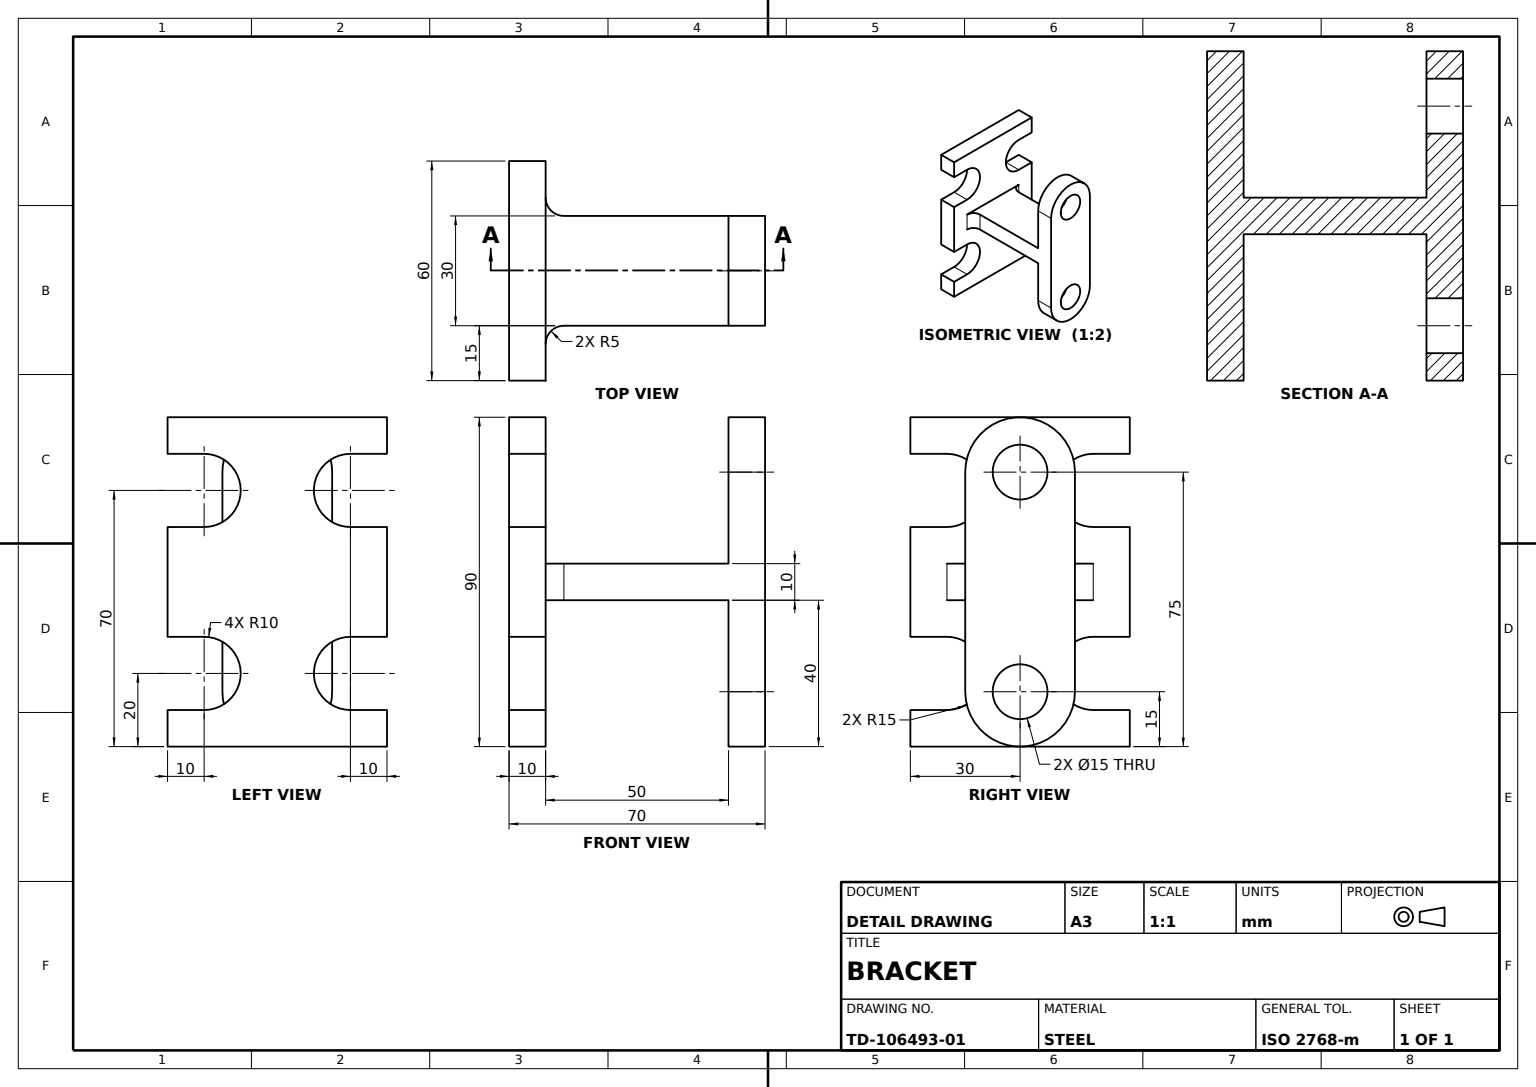
from build123d import *

# Parameters (mm, degrees)
H_BODY_EXTRUDE_60_DEPTH   = 60
RELIEF_CUT_10_DEPTH       = 10
CONNECTOR_ARM_SKETCH_R    = 7.5
CONNECTOR_ARM_BOSS_DEPTH  = 10
NOTCH_CUT_A_SKETCH_W      = 60
NOTCH_CUT_A_SKETCH_H      = 40
NOTCH_CUT_A_DEPTH         = 10
NOTCH_CUT_B_SKETCH_W      = 60
NOTCH_CUT_B_SKETCH_H      = 40
NOTCH_CUT_B_DEPTH         = 10
LINK_PLATE_SKETCH_R       = 7.5
LINK_PLATE_BOSS_DEPTH     = 10
LINK_PLATE_HOLES_SKETCH_W = 50
LINK_PLATE_HOLES_SKETCH_H = 15
LINK_PLATE_HOLES_DEPTH    = 105.880884817
EDGE_FILLETS_R5_R         = 5


with BuildPart() as part:
    # H Profile Sketch → H Body Extrude 60 (new body)
    with BuildSketch(Plane.XY):
        Polygon((0, 0), (0, 45), (10, 45), (10, 5), (50, 5), (50, 45), (60, 45), (60, -45), (50, -45), (50, -5), (10, -5), (10, -45), (0, -45), align=None)
    extrude(amount=H_BODY_EXTRUDE_60_DEPTH)

    # Relief Cut Sketch → Relief Cut 10 (cut)
    with BuildSketch(Plane.ZY):
        with BuildLine():
            Line((10, 35), (0, 35))
            Line((0, 35), (0, 15))
            Line((0, 15), (10, 15))
            ThreePointArc((10, 15), (20, 25), (10, 35))
        make_face()
        with BuildLine():
            Line((60, 15), (60, 35))
            Line((60, 35), (50, 35))
            ThreePointArc((50, 35), (40, 25), (50, 15))
            Line((50, 15), (60, 15))
        make_face()
        with BuildLine():
            Line((10, -15), (0, -15))
            Line((0, -15), (0, -35))
            Line((0, -35), (10, -35))
            ThreePointArc((10, -35), (20, -25), (10, -15))
        make_face()
        with BuildLine():
            Line((60, -35), (60, -15))
            Line((60, -15), (50, -15))
            ThreePointArc((50, -15), (40, -25), (50, -35))
            Line((50, -35), (60, -35))
        make_face()
    extrude(amount=-RELIEF_CUT_10_DEPTH, mode=Mode.SUBTRACT)

    # Connector Arm Sketch → Connector Arm Boss (add)
    with BuildSketch(Plane(origin=(60, 0, 0), x_dir=(0, 0, -1), z_dir=(1, 0, 0))):
        with BuildLine():
            Line((-15, 30), (-15, -30))
            ThreePointArc((-15, -30), (-30, -45), (-45, -30))
            Line((-45, -30), (-45, 30))
            ThreePointArc((-45, 30), (-30, 45), (-15, 30))
        make_face()
        with Locations((-30, 30)):
            Circle(CONNECTOR_ARM_SKETCH_R, mode=Mode.SUBTRACT)
        with Locations((-30, -30)):
            Circle(CONNECTOR_ARM_SKETCH_R, mode=Mode.SUBTRACT)
    extrude(amount=-CONNECTOR_ARM_BOSS_DEPTH)

    # Notch Cut A Sketch → Notch Cut A (cut)
    with BuildSketch(Plane.ZY.offset(-50)):
        with Locations((30, 25)):
            Rectangle(NOTCH_CUT_A_SKETCH_W, NOTCH_CUT_A_SKETCH_H)
    extrude(amount=-NOTCH_CUT_A_DEPTH, mode=Mode.SUBTRACT)

    # Notch Cut B Sketch → Notch Cut B (cut)
    with BuildSketch(Plane.ZY.offset(-50)):
        with Locations((30, -25)):
            Rectangle(NOTCH_CUT_B_SKETCH_W, NOTCH_CUT_B_SKETCH_H)
    extrude(amount=-NOTCH_CUT_B_DEPTH, mode=Mode.SUBTRACT)

    # Link Plate Sketch → Link Plate Boss (add)
    with BuildSketch(Plane(origin=(60, 0, 0), x_dir=(0, 0, -1), z_dir=(1, 0, 0))):
        with BuildLine():
            Line((-15, 30), (-15, -30))
            ThreePointArc((-15, -30), (-30, -45), (-45, -30))
            Line((-45, -30), (-45, 30))
            ThreePointArc((-45, 30), (-30, 45), (-15, 30))
        make_face()
        with Locations((-30, 30)):
            Circle(LINK_PLATE_SKETCH_R, mode=Mode.SUBTRACT)
        with Locations((-30, -30)):
            Circle(LINK_PLATE_SKETCH_R, mode=Mode.SUBTRACT)
    extrude(amount=LINK_PLATE_BOSS_DEPTH)

    # Link Plate Holes Sketch → Link Plate Holes (cut, through all)
    with BuildSketch(Plane(origin=(0, 5, 0), x_dir=(1, 0, 0), z_dir=(0, 1, 0))):
        with Locations((35, -7.5)):
            Rectangle(LINK_PLATE_HOLES_SKETCH_W, LINK_PLATE_HOLES_SKETCH_H)
        with Locations((35, -52.5)):
            Rectangle(LINK_PLATE_HOLES_SKETCH_W, LINK_PLATE_HOLES_SKETCH_H)
    extrude(amount=-LINK_PLATE_HOLES_DEPTH, mode=Mode.SUBTRACT)

    # Edge Fillets R5
    edge_fillets_r5_edges = [part.edges().sort_by_distance(p)[0] for p in [
        (10, 0, 15),
        (10, 0, 45),
    ]]
    fillet(edge_fillets_r5_edges, radius=EDGE_FILLETS_R5_R)


solid = part.part
